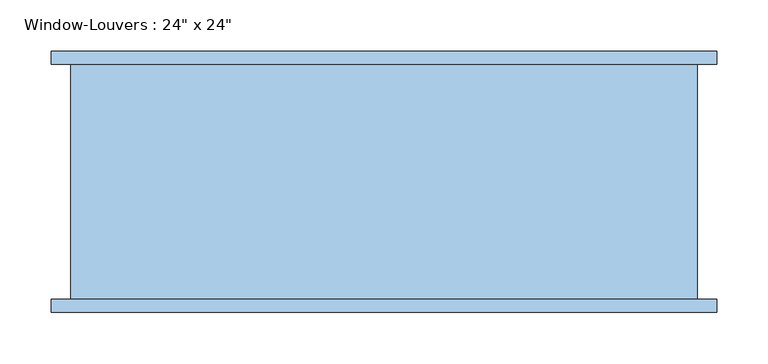
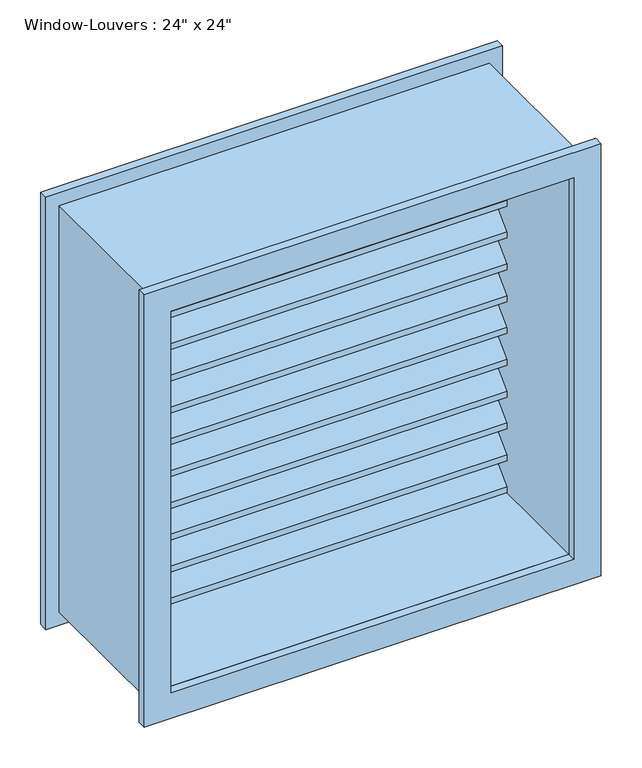
"""IFC4 building model written with IfcOpenShell, lengths in millimetres: window geometry."""

from ifc_helpers import new_model, si_unit, frame, origin, place, context, project, spatial, polyline, outline, extrude, source, transform, mapped, element, save


def window_f2d8fef0(model_context):
    return source(origin(), model_context, "Body", "SweptSolid", [
        extrude(outline(polyline([(107.95, 1419.1754778), (107.95, 1410.1952217), (69.85, 1448.2952217), (31.75, 1410.1952217), (31.75, 1419.1754778), (69.85, 1457.2754778), (107.95, 1419.1754778)])), frame((-285.75, 0.0, 0.0), z_axis=(1.0, 0.0, 0.0), x_axis=(0.0, 1.0, 0.0)), (0.0, 0.0, 1.0), 571.5),
        extrude(outline(polyline([(107.95, 1371.5009557), (107.95, 1362.5206995), (69.85, 1400.6206995), (31.75, 1362.5206995), (31.75, 1371.5009557), (69.85, 1409.6009557), (107.95, 1371.5009557)])), frame((-285.75, 0.0, 0.0), z_axis=(1.0, 0.0, 0.0), x_axis=(0.0, 1.0, 0.0)), (0.0, 0.0, 1.0), 571.5),
        extrude(outline(polyline([(107.95, 1323.8264335), (107.95, 1314.8461774), (69.85, 1352.9461774), (31.75, 1314.8461774), (31.75, 1323.8264335), (69.85, 1361.9264335), (107.95, 1323.8264335)])), frame((-285.75, 0.0, 0.0), z_axis=(1.0, 0.0, 0.0), x_axis=(0.0, 1.0, 0.0)), (0.0, 0.0, 1.0), 571.5),
        extrude(outline(polyline([(107.95, 1276.1519113), (107.95, 1267.1716552), (69.85, 1305.2716552), (31.75, 1267.1716552), (31.75, 1276.1519113), (69.85, 1314.2519113), (107.95, 1276.1519113)])), frame((-285.75, 0.0, 0.0), z_axis=(1.0, 0.0, 0.0), x_axis=(0.0, 1.0, 0.0)), (0.0, 0.0, 1.0), 571.5),
        extrude(outline(polyline([(107.95, 1228.4773891), (107.95, 1219.497133), (69.85, 1257.597133), (31.75, 1219.497133), (31.75, 1228.4773891), (69.85, 1266.5773891), (107.95, 1228.4773891)])), frame((-285.75, 0.0, 0.0), z_axis=(1.0, 0.0, 0.0), x_axis=(0.0, 1.0, 0.0)), (0.0, 0.0, 1.0), 571.5),
        extrude(outline(polyline([(107.95, 1180.802867), (107.95, 1171.8226109), (69.85, 1209.9226109), (31.75, 1171.8226109), (31.75, 1180.802867), (69.85, 1218.902867), (107.95, 1180.802867)])), frame((-285.75, 0.0, 0.0), z_axis=(1.0, 0.0, 0.0), x_axis=(0.0, 1.0, 0.0)), (0.0, 0.0, 1.0), 571.5),
        extrude(outline(polyline([(107.95, 1133.1283448), (107.95, 1124.1480887), (69.85, 1162.2480887), (31.75, 1124.1480887), (31.75, 1133.1283448), (69.85, 1171.2283448), (107.95, 1133.1283448)])), frame((-285.75, 0.0, 0.0), z_axis=(1.0, 0.0, 0.0), x_axis=(0.0, 1.0, 0.0)), (0.0, 0.0, 1.0), 571.5),
        extrude(outline(polyline([(107.95, 1085.4538226), (107.95, 1076.4735665), (69.85, 1114.5735665), (31.75, 1076.4735665), (31.75, 1085.4538226), (69.85, 1123.5538226), (107.95, 1085.4538226)])), frame((-285.75, 0.0, 0.0), z_axis=(1.0, 0.0, 0.0), x_axis=(0.0, 1.0, 0.0)), (0.0, 0.0, 1.0), 571.5),
        extrude(outline(polyline([(107.95, 1037.7793005), (107.95, 1028.7990443), (69.85, 1066.8990443), (31.75, 1028.7990443), (31.75, 1037.7793005), (69.85, 1075.8793005), (107.95, 1037.7793005)])), frame((-285.75, 0.0, 0.0), z_axis=(1.0, 0.0, 0.0), x_axis=(0.0, 1.0, 0.0)), (0.0, 0.0, 1.0), 571.5),
        extrude(outline(polyline([(107.95, 990.1047783), (107.95, 981.1245222), (69.85, 1019.2245222), (31.75, 981.1245222), (31.75, 990.1047783), (69.85, 1028.2047783), (107.95, 990.1047783)])), frame((-285.75, 0.0, 0.0), z_axis=(1.0, 0.0, 0.0), x_axis=(0.0, 1.0, 0.0)), (0.0, 0.0, 1.0), 571.5),
        extrude(outline(polyline([(107.95, 1466.85), (107.95, 1457.8697439), (69.85, 1495.9697439), (31.75, 1457.8697439), (31.75, 1466.85), (69.85, 1504.95), (107.95, 1466.85)])), frame((-285.75, 0.0, 0.0), z_axis=(1.0, 0.0, 0.0), x_axis=(0.0, 1.0, 0.0)), (0.0, 0.0, 1.0), 571.5),
        extrude(outline(polyline([(107.95, 942.4302561), (107.95, 933.45), (69.85, 971.55), (31.75, 933.45), (31.75, 942.4302561), (69.85, 980.5302561), (107.95, 942.4302561)])), frame((-285.75, 0.0, 0.0), z_axis=(1.0, 0.0, 0.0), x_axis=(0.0, 1.0, 0.0)), (0.0, 0.0, 1.0), 571.5),
        extrude(outline(polyline([(1524.0, 304.8), (1524.0, -304.8), (914.4, -304.8), (914.4, 304.8), (1524.0, 304.8)]), holes=[polyline([(1504.95, 285.75), (933.45, 285.75), (933.45, -285.75), (1504.95, -285.75), (1504.95, 285.75)])]), frame((0.0, -120.65, 0.0), z_axis=(0.0, 1.0, 0.0), x_axis=(0.0, 0.0, 1.0)), (0.0, 0.0, 1.0), 228.6),
        extrude(outline(polyline([(1543.05, 323.85), (1543.05, -323.85), (895.35, -323.85), (895.35, 323.85), (1543.05, 323.85)]), holes=[polyline([(1504.95, 285.75), (933.45, 285.75), (933.45, -285.75), (1504.95, -285.75), (1504.95, 285.75)])]), frame((0.0, -133.35, 0.0), z_axis=(0.0, 1.0, 0.0), x_axis=(0.0, 0.0, 1.0)), (0.0, 0.0, 1.0), 12.7),
        extrude(outline(polyline([(1543.05, -323.85), (895.35, -323.85), (895.35, 323.85), (1543.05, 323.85), (1543.05, -323.85)]), holes=[polyline([(1504.95, -285.75), (1504.95, 285.75), (933.45, 285.75), (933.45, -285.75), (1504.95, -285.75)])]), frame((0.0, 107.95, 0.0), z_axis=(0.0, 1.0, 0.0), x_axis=(0.0, 0.0, 1.0)), (0.0, 0.0, 1.0), 12.7),
    ])


if __name__ == "__main__":
    model = new_model("IFC4")
    model_context = context("Model", 3, world=origin())
    ifc_project = project(units=[si_unit("LENGTHUNIT", "METRE", prefix="MILLI")], contexts=[model_context])
    site = spatial("IfcSite", under=ifc_project)
    building = spatial("IfcBuilding", under=site)
    placement = place(None, origin())
    window_shape = window_f2d8fef0(model_context)
    element("IfcWindow", 1, ObjectType="Window-Louvers : 24\" x 24\"", at=placement, inside=building, context=model_context, shape_type="MappedRepresentation", body=[
        mapped(window_shape, transform((0.0, 0.0, 0.0), x_axis=(1.0, 0.0, 0.0), y_axis=(0.0, 1.0, 0.0), z_axis=(0.0, 0.0, 1.0))),
    ])
    save(model, "model.ifc")

# Revit data of these elements
# Type "Window-Louvers : 24\" x 24\""
#   Type Mark = "22"
#   Construction Type Id = "GSP4R"
#   Assembly Code = "B20"
#   Analytic Construction = "1/8 in Pilkington single glazing"
#   Visual Light Transmittance = 0.9
#   Thermal Resistance (R) = 1.53941 (h·ft²·°F)/BTU
#   Solar Heat Gain Coefficient = 0.78
#   Max Height = 1' - 11.74264"
#   Height = 2' - 0"
#   Heat Transfer Coefficient (U) = 0.6496 BTU/(h·ft²·°F)
#   Blade Width [instance default] = 1' - 10 1/2"
#   Blade Vertical Thickness = 0' - 0.35355"
#   Blade Thickness = 0' - 0 1/4"
#   Blade Spacing = 0' - 1 1/2"
#   Blade Height = 0' - 1.85355"
#   Blade Depth = 0' - 3"
#   Blade Angle = 45.00°
#   Default Sill Height = 3' - 0"
#   Trim Projection_Exterior = 0' - 0 1/2"
#   Trim Projection_Interior = 0' - 0 1/2"
#   Trim Width_Exterior = 0' - 1 1/2"
#   Trim Width_Interior = 0' - 1 1/2"
#   Width = 2' - 0"
#   Max Blade Count = 12
#   Define Thermal Properties by = 1
#   Blade Count = 12
#   Frame Material = Birch
#   Louver Material = Birch
#   Trim Exterior Material = Birch
#   Trim Interior Material = Birch
#   Wall Closure = (empty or 0)
# Element 1 (IfcWindow, "Window-Louvers : 24\" x 24\"")
#   Materials on its faces: "Birch"
# Materials
#   "Birch": class "Wood", colour RGB 224 178 126, transparency 0, Description = "Betula Alleghaniensis", Cost = 0
